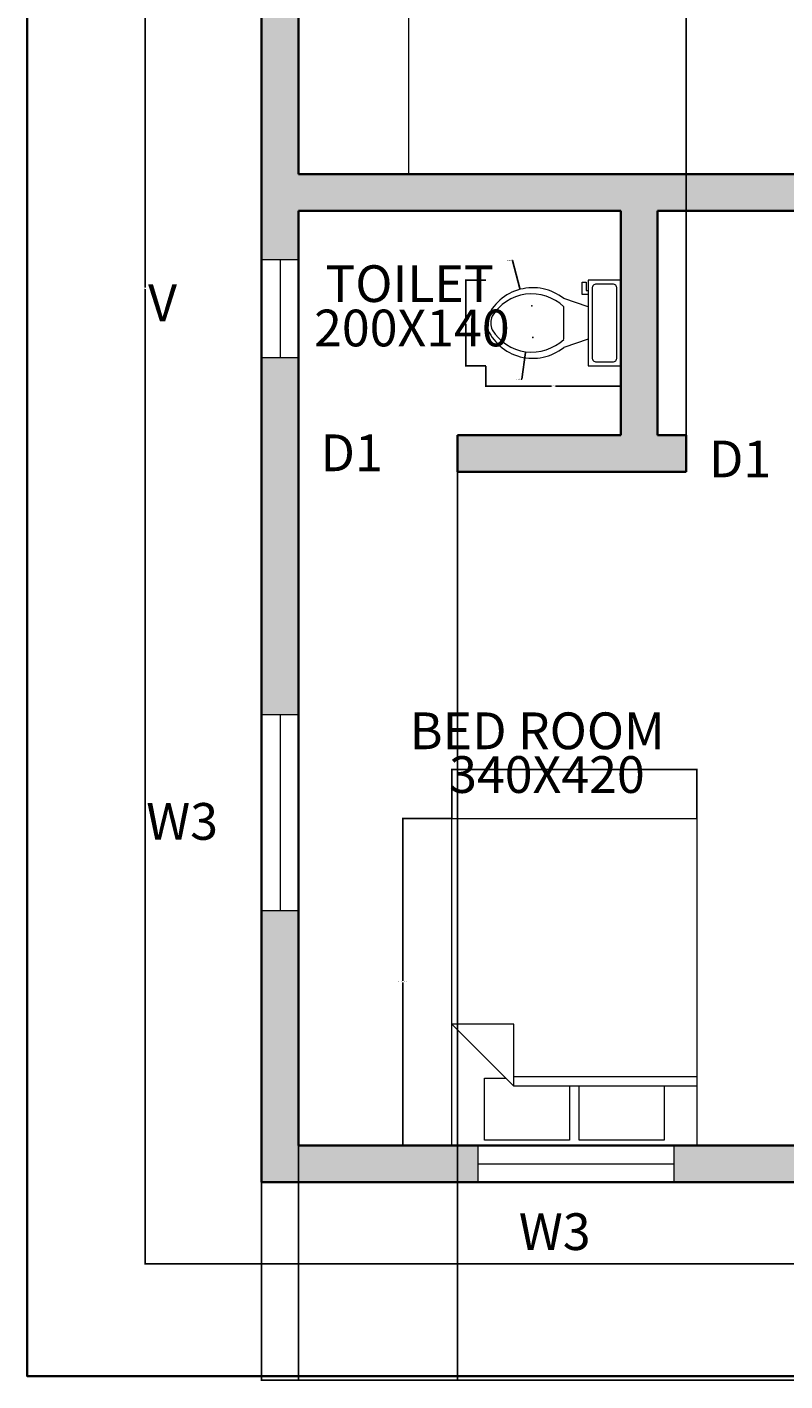
# Model space of a CAD drawing. Units: inches. Extents: x 1332 to 3175, y 1481 to 2088.
# Tile 1 of 5: x 1332 to 1518, y 1484 to 1816. Entities that reach past the tile are written whole.
import ezdxf

# ---------------------------------------------------------------- set-up
doc = ezdxf.new("R2010")
doc.units = ezdxf.units.IN
for name, color, linetype, lineweight in [('A-ANNO-DIMS', 2, 'Continuous', 18), ('A-ANNO-TEXT', 7, 'Continuous', 18), ('A-ANNO-TTLB', 7, 'Continuous', 35), ('A-AREA-IDEN', 7, 'Continuous', 18), ('A-FLOR-CASE', 8, 'Continuous', 18), ('A-FLOR-FIXT', 8, 'Continuous', 18), ('A-FURN', 8, 'Continuous', 18), ('A-WALL', 7, 'Continuous', 35)]:
    doc.layers.add(name, color=color, linetype=linetype, lineweight=lineweight)
doc.layers.add('A-GLAZ', color=30, linetype='Continuous', lineweight=18, true_color=0xf8991e)
doc.layers.add('A-WALL-PATT', color=18, linetype='Continuous', lineweight=13, true_color=0x000000)
doc.styles.get("Standard").update_dxf_attribs({"font": 'arial.ttf'})
doc.dimstyles.get("Standard").update_dxf_attribs({"dimtxt": 0.18, "dimasz": 0.18, "dimexe": 0.18, "dimexo": 0.0625, "dimgap": 0.09, "dimtad": 0, "dimtih": 1, "dimtoh": 1, "dimdec": 4, "dimzin": 0, "dimdsep": 46, "dimtxsty": 'Standard', "dimcen": 0.09, "dimadec": 0, "dimazin": 0, "dimtfac": 1, "dimtdec": 4, "dimtofl": 0, "dimtmove": 0, "dimatfit": 3, "dimfxl": 1, "dimtolj": 1, "dimtzin": 0, "dimarcsym": 0})

# ---------------------------------------------------------------- blocks, each defined once
blk = doc.blocks.new('Bed - Queen')
for p, q in [((0, -80.00003), (0, 0)), ((0, 0), (59.99999, 0)), ((59.99999, 0), (59.99999, -80.00003)), ((7.99999, -1.2), (28.79998, -1.2)), ((7.99999, -14.4), (7.99999, -1.2)), ((28.79998, -1.2), (28.79998, -14.4)), ((31.19999, -1.2), (51.99999, -1.2)), ((31.19999, -14.4), (31.19999, -1.2)), ((51.99999, -1.2), (51.99999, -16.4)), ((0, -14.4), (44.8, -14.4)), ((59.99999, -29.6), (44.8, -14.4)), ((44.8, -14.4), (44.8, -29.6)), ((51.99999, -16.4), (46.79936, -16.4)), ((44.8, -16.8), (0, -16.8)), ((44.8, -29.6), (59.99999, -29.6)), ((59.99999, -80.00003), (0, -80.00003))]:
    blk.add_line(p, q)
blk = doc.blocks.new('Toilet - top')
for p, q in [((9.5, -6), (9.5, -2)), ((-10, -8.5), (-8, -8.5)), ((-10, -9.5), (-10, -8.5)), ((-7, -9.5), (-10, -9.5)), ((-8, -8.5), (-8, -8)), ((-7, -8), (-7, -9.5)), ((-4, -8), (-6, -14)), ((4, -8), (6, -14)), ((4, -14), (-4, -14))]:
    blk.add_line(p, q)
blk.add_lwpolyline([(10.5, -8), (10.5, 0), (-10.5, 0), (-10.5, -8)], close=True)
for points in [[(-9.5, -2), (-9.5, -6)], [(8.5, -1), (-8.5, -1)], [(-8.5, -7), (8.5, -7)]]:
    blk.add_lwpolyline(points)
for centre, radius, start, end in [((-8.62, -1.88), 0.884, 81.8699, 188.1301), ((8.62, -1.88), 0.884, 351.8699, 98.1301), ((-8.62, -6.12), 0.884, 171.8699, 278.1301), ((8.62, -6.12), 0.884, 261.8699, 8.1301), ((3.52, -21.58), 12.17, 141.4691, 247.9714), ((4.2, -21.82), 11.33, 136.3677, 238.9468), ((-3.52, -21.58), 12.17, 292.0284, 38.5307), ((-4.2, -21.82), 11.33, 301.053, 43.6321), ((0, -27.88), 4, 245.7318, 294.2682), ((0, -29), 4, 254.8605, 285.1395)]:
    blk.add_arc(centre, radius, start, end)
blk = doc.blocks.new('WIN-W3-48')
for p, q in [((0, 9), (0, 0)), ((48, 9), (48, 0)), ((0, 4.5), (48, 4.5))]:
    blk.add_line(p, q)
blk = doc.blocks.new('VENT-24')
for p, q in [((0, 9), (0, 0)), ((24, 9), (24, 0)), ((0, 4.5), (24, 4.5))]:
    blk.add_line(p, q)
blk = doc.blocks.new('*D19')
at = {"layer": 'A-ANNO-DIMS', "color": 0, "lineweight": -2, "transparency": 16777216}
for p, q in [((1436.18, 1622.23), (1424.06, 1622.23)), ((1424.24, 1622.05), (1424.24, 1582.42)), ((1424.24, 1542.41), (1424.24, 1582.04)), ((1436.18, 1542.23), (1424.06, 1542.23))]:
    blk.add_line(p, q, dxfattribs=at)
at = {"layer": 'A-ANNO-DIMS', "color": 0, "transparency": 16777216}
for points in [[(1424.21, 1622.05), (1424.27, 1622.05), (1424.24, 1622.23)], [(1424.21, 1542.41), (1424.27, 1542.41), (1424.24, 1542.23)]]:
    blk.add_solid(points, dxfattribs=at)
at = {"layer": 'Defpoints', "color": 0, "transparency": 16777216}
for p in [(1436.24, 1622.23), (1424.24, 1542.23), (1436.24, 1542.23)]:
    blk.add_point(p, dxfattribs=at)
at = {"layer": 'A-ANNO-DIMS', "color": 0, "transparency": 16777216, "insert": (1424.24, 1582.23), "char_height": 0.18, "attachment_point": 5}
blk.add_mtext('\\A1;QUEEN BED 80 TYP.', dxfattribs=at)
blk = doc.blocks.new('*D20')
at = {"layer": 'A-ANNO-DIMS', "color": 0, "lineweight": -2, "transparency": 16777216}
for p, q in [((1436.24, 1622.29), (1436.24, 1634.41)), ((1436.42, 1634.23), (1465.72, 1634.23)), ((1496.06, 1634.23), (1466.77, 1634.23)), ((1496.24, 1622.29), (1496.24, 1634.41))]:
    blk.add_line(p, q, dxfattribs=at)
at = {"layer": 'A-ANNO-DIMS', "color": 0, "transparency": 16777216}
for points in [[(1436.42, 1634.26), (1436.42, 1634.2), (1436.24, 1634.23)], [(1496.06, 1634.26), (1496.06, 1634.2), (1496.24, 1634.23)]]:
    blk.add_solid(points, dxfattribs=at)
at = {"layer": 'Defpoints', "color": 0, "transparency": 16777216}
for p in [(1436.24, 1634.23), (1436.24, 1622.23), (1496.24, 1622.23)]:
    blk.add_point(p, dxfattribs=at)
at = {"layer": 'A-ANNO-DIMS', "color": 0, "transparency": 16777216, "insert": (1466.24, 1634.23), "char_height": 0.18, "attachment_point": 5}
blk.add_mtext('\\A1;60 TYP.', dxfattribs=at)
blk = doc.blocks.new('*D35')
at = {"layer": 'A-ANNO-DIMS', "color": 0, "lineweight": -2, "transparency": 16777216}
for p, q in [((1444.59, 1733.06), (1444.59, 1727.98)), ((1477.63, 1733.06), (1477.63, 1727.98)), ((1444.77, 1728.16), (1460.64, 1728.16)), ((1477.45, 1728.16), (1461.58, 1728.16))]:
    blk.add_line(p, q, dxfattribs=at)
at = {"layer": 'A-ANNO-DIMS', "color": 0, "transparency": 16777216}
for points in [[(1444.77, 1728.19), (1444.77, 1728.13), (1444.59, 1728.16)], [(1477.45, 1728.19), (1477.45, 1728.13), (1477.63, 1728.16)]]:
    blk.add_solid(points, dxfattribs=at)
at = {"layer": 'Defpoints', "color": 0, "transparency": 16777216}
for p in [(1444.59, 1733.12), (1477.63, 1733.12), (1477.63, 1728.16)]:
    blk.add_point(p, dxfattribs=at)
at = {"layer": 'A-ANNO-DIMS', "color": 0, "transparency": 16777216, "insert": (1461.11, 1728.16), "char_height": 0.18, "attachment_point": 5}
blk.add_mtext('\\A1;WC 33', dxfattribs=at)
blk = doc.blocks.new('*D36')
at = {"layer": 'A-ANNO-DIMS', "color": 0, "lineweight": -2, "transparency": 16777216}
for p, q in [((1444.52, 1754.12), (1439.45, 1754.12)), ((1439.63, 1753.94), (1439.63, 1743.8)), ((1439.63, 1733.3), (1439.63, 1743.44)), ((1444.52, 1733.12), (1439.45, 1733.12))]:
    blk.add_line(p, q, dxfattribs=at)
at = {"layer": 'A-ANNO-DIMS', "color": 0, "transparency": 16777216}
for points in [[(1439.6, 1753.94), (1439.66, 1753.94), (1439.63, 1754.12)], [(1439.6, 1733.3), (1439.66, 1733.3), (1439.63, 1733.12)]]:
    blk.add_solid(points, dxfattribs=at)
at = {"layer": 'Defpoints', "color": 0, "transparency": 16777216}
for p in [(1444.59, 1754.12), (1439.63, 1733.12), (1444.59, 1733.12)]:
    blk.add_point(p, dxfattribs=at)
at = {"layer": 'A-ANNO-DIMS', "color": 0, "transparency": 16777216, "insert": (1439.63, 1743.62), "char_height": 0.18, "attachment_point": 5}
blk.add_mtext('\\A1;21', dxfattribs=at)
blk = doc.blocks.new('*D37')
at = {"layer": 'A-ANNO-DIMS', "color": 0, "lineweight": -2, "transparency": 16777216}
for p, q in [((1851.13, 1589.06), (1851.13, 1484.44)), ((1389.63, 1533.06), (1389.63, 1484.44)), ((1389.81, 1484.62), (1619.98, 1484.62)), ((1850.95, 1484.62), (1620.78, 1484.62))]:
    blk.add_line(p, q, dxfattribs=at)
at = {"layer": 'A-ANNO-DIMS', "color": 0, "transparency": 16777216}
for points in [[(1389.81, 1484.65), (1389.81, 1484.59), (1389.63, 1484.62)], [(1850.95, 1484.65), (1850.95, 1484.59), (1851.13, 1484.62)]]:
    blk.add_solid(points, dxfattribs=at)
at = {"layer": 'Defpoints', "color": 0, "transparency": 16777216}
for p in [(1851.13, 1589.12), (1389.63, 1533.12), (1851.13, 1484.62)]:
    blk.add_point(p, dxfattribs=at)
at = {"layer": 'A-ANNO-DIMS', "color": 0, "transparency": 16777216, "insert": (1620.38, 1484.62), "char_height": 0.18, "attachment_point": 5}
blk.add_mtext('\\A1;461.5', dxfattribs=at)
blk = doc.blocks.new('*D38')
at = {"layer": 'A-ANNO-DIMS', "color": 0, "lineweight": -2, "transparency": 16777216}
for p, q in [((1444.57, 1991.12), (1360.95, 1991.12)), ((1361.13, 1990.94), (1361.13, 1752.3)), ((1361.13, 1513.3), (1361.13, 1751.94)), ((1532.57, 1513.12), (1360.95, 1513.12))]:
    blk.add_line(p, q, dxfattribs=at)
at = {"layer": 'A-ANNO-DIMS', "color": 0, "transparency": 16777216}
for points in [[(1361.1, 1990.94), (1361.16, 1990.94), (1361.13, 1991.12)], [(1361.1, 1513.3), (1361.16, 1513.3), (1361.13, 1513.12)]]:
    blk.add_solid(points, dxfattribs=at)
at = {"layer": 'Defpoints', "color": 0, "transparency": 16777216}
for p in [(1361.13, 1991.12), (1444.63, 1991.12), (1532.63, 1513.12)]:
    blk.add_point(p, dxfattribs=at)
at = {"layer": 'A-ANNO-DIMS', "color": 0, "transparency": 16777216, "insert": (1361.13, 1752.12), "char_height": 0.18, "attachment_point": 5}
blk.add_mtext('\\A1;478', dxfattribs=at)
blk = doc.blocks.new('*D86')
at = {"layer": 'A-ANNO-DIMS', "color": 0, "lineweight": -2, "transparency": 16777216}
for p, q in [((1398.63, 1735.06), (1398.63, 1484.44)), ((1437.63, 1716.06), (1437.63, 1484.44)), ((1398.81, 1484.62), (1417.91, 1484.62)), ((1437.45, 1484.62), (1418.35, 1484.62))]:
    blk.add_line(p, q, dxfattribs=at)
at = {"layer": 'A-ANNO-DIMS', "color": 0, "transparency": 16777216}
for points in [[(1398.81, 1484.65), (1398.81, 1484.59), (1398.63, 1484.62)], [(1437.45, 1484.65), (1437.45, 1484.59), (1437.63, 1484.62)]]:
    blk.add_solid(points, dxfattribs=at)
at = {"layer": 'Defpoints', "color": 0, "transparency": 16777216}
for p in [(1398.63, 1735.12), (1437.63, 1716.12), (1437.63, 1484.62)]:
    blk.add_point(p, dxfattribs=at)
at = {"layer": 'A-ANNO-DIMS', "color": 0, "transparency": 16777216, "insert": (1418.13, 1484.62), "char_height": 0.18, "attachment_point": 5}
blk.add_mtext('\\A1;39', dxfattribs=at)
blk = doc.blocks.new('*D87')
at = {"layer": 'A-ANNO-DIMS', "color": 0, "lineweight": -2, "transparency": 16777216}
for p, q in [((1493.63, 1716.18), (1493.63, 2019.8)), ((1493.81, 2019.62), (1512.91, 2019.62)), ((1532.45, 2019.62), (1513.35, 2019.62)), ((1532.63, 1716.18), (1532.63, 2019.8))]:
    blk.add_line(p, q, dxfattribs=at)
at = {"layer": 'A-ANNO-DIMS', "color": 0, "transparency": 16777216}
for points in [[(1493.81, 2019.65), (1493.81, 2019.59), (1493.63, 2019.62)], [(1532.45, 2019.65), (1532.45, 2019.59), (1532.63, 2019.62)]]:
    blk.add_solid(points, dxfattribs=at)
at = {"layer": 'Defpoints', "color": 0, "transparency": 16777216}
for p in [(1532.63, 2019.62), (1493.63, 1716.12), (1532.63, 1716.12)]:
    blk.add_point(p, dxfattribs=at)
at = {"layer": 'A-ANNO-DIMS', "color": 0, "transparency": 16777216, "insert": (1513.13, 2019.62), "char_height": 0.18, "attachment_point": 5}
blk.add_mtext('\\A1;39', dxfattribs=at)
blk = doc.blocks.new('*D92')
at = {"layer": 'A-ANNO-DIMS', "color": 0, "lineweight": -2, "transparency": 16777216}
for p, q in [((1450.92, 1758.93), (1451.1, 1758.93)), ((1451.1, 1758.93), (1452.91, 1752.04)), ((1455.96, 1740.1), (1456.14, 1740.1)), ((1456.05, 1740.01), (1456.05, 1740.19))]:
    blk.add_line(p, q, dxfattribs=at)
at = {"layer": 'A-ANNO-DIMS', "color": 0, "transparency": 16777216}
blk.add_solid([(1452.94, 1752.05), (1452.88, 1752.03), (1452.96, 1751.87)], dxfattribs=at)
at = {"layer": 'Defpoints', "color": 0, "transparency": 16777216}
for p in [(1452.96, 1751.87), (1456.05, 1740.1)]:
    blk.add_point(p, dxfattribs=at)
at = {"layer": 'A-ANNO-DIMS', "color": 0, "transparency": 16777216, "insert": (1450.25, 1758.93), "char_height": 0.18, "attachment_point": 5}
blk.add_mtext('\\A1;2X R12.17', dxfattribs=at)
blk = doc.blocks.new('*D93')
at = {"layer": 'A-ANNO-DIMS', "color": 0, "lineweight": -2, "transparency": 16777216}
for p, q in [((1455.72, 1747.82), (1455.9, 1747.82)), ((1455.81, 1747.73), (1455.81, 1747.91)), ((1453.4, 1729.85), (1454.28, 1736.41)), ((1453.22, 1729.85), (1453.4, 1729.85))]:
    blk.add_line(p, q, dxfattribs=at)
at = {"layer": 'A-ANNO-DIMS', "color": 0, "transparency": 16777216}
blk.add_solid([(1454.25, 1736.42), (1454.31, 1736.41), (1454.3, 1736.59)], dxfattribs=at)
at = {"layer": 'Defpoints', "color": 0, "transparency": 16777216}
for p in [(1455.81, 1747.82), (1454.3, 1736.59)]:
    blk.add_point(p, dxfattribs=at)
at = {"layer": 'A-ANNO-DIMS', "color": 0, "transparency": 16777216, "insert": (1452.54, 1729.85), "char_height": 0.18, "attachment_point": 5}
blk.add_mtext('\\A1;2X R11.33', dxfattribs=at)

msp = doc.modelspace()

# ---------------------------------------------------------------- hatches: boundary and pattern name
at = {"layer": 'A-WALL-PATT'}
h = msp.add_hatch(color=256, dxfattribs=at)
h.dxf.hatch_style = 1
h.paths.add_polyline_path([(1398.6316, 1914.1183), (1442.6316, 1914.1183), (1442.6316, 1923.1183), (1389.6316, 1923.1183), (1389.6316, 1868.1183), (1398.6316, 1868.1183)])
h.paths.add_polyline_path([(1398.6316, 1828.1183), (1389.6316, 1828.1183), (1389.6316, 1759.1183), (1398.6316, 1759.1183), (1398.6316, 1771.1183), (1477.6316, 1771.1183), (1477.6316, 1716.1183), (1437.6316, 1716.1183), (1437.6316, 1707.1183), (1493.6316, 1707.1183), (1493.6316, 1716.1183), (1486.6316, 1716.1183), (1486.6316, 1771.1183), (1532.6316, 1771.1183), (1532.6316, 1780.1183), (1398.6316, 1780.1183)])
h.paths.add_polyline_path([(1398.6316, 1735.1183), (1389.6316, 1735.1183), (1389.6316, 1647.6183), (1398.6316, 1647.6183)])
h.paths.add_polyline_path([(1398.6316, 1599.6183), (1389.6316, 1599.6183), (1389.6316, 1533.1183), (1442.6316, 1533.1183), (1442.6316, 1542.1183), (1398.6316, 1542.1183)])
h.paths.add_polyline_path([(1541.6316, 1589.1183), (1576.5616, 1589.1183), (1576.5616, 1598.1183), (1541.6316, 1598.1183), (1541.6316, 1707.1183), (1576.5616, 1707.1183), (1576.5616, 1716.1183), (1532.6316, 1716.1183), (1532.6316, 1542.1183), (1490.6316, 1542.1183), (1490.6316, 1533.1183), (1541.6316, 1533.1183)])
h.paths.add_polyline_path([(1717.1316, 1707.1183), (1752.1316, 1707.1183), (1752.1316, 1716.1183), (1672.5616, 1716.1183), (1672.5616, 1707.1183), (1708.1316, 1707.1183), (1708.1316, 1598.1183), (1672.5616, 1598.1183), (1672.5616, 1589.1183), (1717.1316, 1589.1183)])
h.paths.add_polyline_path([(1851.1316, 1761.1183), (1842.1316, 1761.1183), (1842.1316, 1716.1183), (1800.1316, 1716.1183), (1800.1316, 1707.1183), (1851.1316, 1707.1183)])
h.paths.add_polyline_path([(1851.1316, 1855.1183), (1784.1316, 1855.1183), (1784.1316, 1923.1183), (1750.1316, 1923.1183), (1750.1316, 1914.1183), (1775.1316, 1914.1183), (1775.1316, 1855.1183), (1750.1316, 1855.1183), (1750.1316, 1846.1183), (1842.1316, 1846.1183), (1842.1316, 1801.1183), (1851.1316, 1801.1183)])
h.paths.add_polyline_path([(1717.1316, 1914.1183), (1726.1316, 1914.1183), (1726.1316, 1923.1183), (1673.1316, 1923.1183), (1673.1316, 1914.1183), (1708.1316, 1914.1183), (1708.1316, 1755.1183), (1717.1316, 1755.1183)])
h.paths.add_polyline_path([(1661.1316, 1855.1183), (1636.1316, 1855.1183), (1636.1316, 1914.1183), (1649.1316, 1914.1183), (1649.1316, 1923.1183), (1611.3665, 1923.1183), (1611.3665, 1914.1183), (1627.1316, 1914.1183), (1627.1316, 1846.1183), (1661.1316, 1846.1183)])
h.paths.add_polyline_path([(1541.6316, 1914.1183), (1563.3665, 1914.1183), (1563.3665, 1923.1183), (1541.6316, 1923.1183), (1541.6316, 1991.1183), (1528.6316, 1991.1183), (1528.6316, 1982.1183), (1532.6316, 1982.1183), (1532.6316, 1914.1183), (1532.6316, 1816.1183), (1541.6316, 1816.1183)])
h.paths.add_polyline_path([(1453.6316, 1982.1183), (1457.6316, 1982.1183), (1457.6316, 1991.1183), (1444.6316, 1991.1183), (1444.6316, 1956.1183), (1453.6316, 1956.1183)])

# ---------------------------------------------------------------- linework, layer by layer
at = {"layer": 'A-ANNO-TTLB'}
msp.add_lwpolyline([(1332.1674, 2088.4777), (3159.6908, 2088.4777), (3159.6908, 1485.6439), (1332.1674, 1485.6439)], close=True, dxfattribs=at)
at = {"layer": 'A-FLOR-CASE'}
msp.add_line((1425.7005, 1780.1183), (1425.7005, 1891.601), dxfattribs=at)
at = {"layer": 'A-WALL'}
for p, q in [((1389.6316, 1923.1183), (1389.6316, 1533.1183)), ((1398.6316, 1914.1183), (1398.6316, 1780.1183)), ((1398.6316, 1780.1183), (1532.6316, 1780.1183)), ((1398.6316, 1771.1183), (1477.6316, 1771.1183)), ((1398.6316, 1771.1183), (1398.6316, 1542.1183)), ((1477.6316, 1771.1183), (1477.6316, 1716.1183)), ((1486.6316, 1771.1183), (1486.6316, 1716.1183)), ((1486.6316, 1771.1183), (1532.6316, 1771.1183)), ((1437.6316, 1716.1183), (1477.6316, 1716.1183)), ((1437.6316, 1716.1183), (1477.6316, 1716.1183)), ((1437.6316, 1716.1183), (1437.6316, 1707.1183)), ((1486.6316, 1716.1183), (1493.6316, 1716.1183)), ((1486.6316, 1716.1183), (1493.6316, 1716.1183)), ((1493.6316, 1716.1183), (1493.6316, 1707.1183)), ((1437.6316, 1707.1183), (1493.6316, 1707.1183)), ((1398.6316, 1542.1183), (1532.6316, 1542.1183)), ((1389.6316, 1533.1183), (1541.6316, 1533.1183))]:
    msp.add_line(p, q, dxfattribs=at)

# ---------------------------------------------------------------- block references
at = {"layer": 'A-FLOR-FIXT', "rotation": 270}
msp.add_blockref('Toilet - top', (1477.6316, 1743.6183), dxfattribs=at)
at = {"layer": 'A-FURN', "rotation": 180}
msp.add_blockref('Bed - Queen', (1496.2447, 1542.2313), dxfattribs=at)
at = {"layer": 'A-GLAZ'}
for name, p, rotation in [('VENT-24', (1389.6316, 1759.1183), 270.0000000000015), ('WIN-W3-48', (1389.6316, 1647.6183), 270.0000000000006)]:
    msp.add_blockref(name, p, dxfattribs=dict(at, rotation=rotation))
msp.add_blockref('WIN-W3-48', (1442.6316, 1533.1183), dxfattribs=at)

# ---------------------------------------------------------------- texts
at = {"layer": 'A-ANNO-TEXT'}
for s, p in [('      V', (1345.3144, 1744.0608)), ('      D1', (1387.5429, 1707.3201)), ('      D1', (1482.7043, 1705.8048)), ('    W3', (1350.3492, 1617.0164)), ('    W3', (1441.6235, 1516.511))]:
    msp.add_text(s, height=9, dxfattribs=at).set_placement(p)
at = {"layer": 'A-AREA-IDEN'}
for s, p in [(' TOILET', (1402.4712, 1748.759)), ('200X140', (1402.4712, 1737.8945)), ('BED ROOM', (1425.8978, 1639.2106)), ('340X420', (1435.5603, 1628.4969))]:
    msp.add_text(s, height=9, dxfattribs=at).set_placement(p)

# ---------------------------------------------------------------- dimensions: what is measured, and where the dimension line sits
at = {"layer": 'A-ANNO-DIMS'}
for base, p1, p2, override, picture, middle in [((1532.6316, 2019.6183), (1493.6316, 1716.1183), (1532.6316, 1716.1183), {"dimdec": 0, "dimlfac": 1, "dimrnd": 0, "dimzin": 0, "dimdsep": 46, "dimlunit": 2}, '*D87', (1513.1316, 2019.6183)), ((1437.6316, 1484.6183), (1398.6316, 1735.1183), (1437.6316, 1716.1183), {"dimdec": 0, "dimlfac": 1, "dimrnd": 0, "dimzin": 0, "dimdsep": 46, "dimlunit": 2}, '*D86', (1418.1316, 1484.6183)), ((1851.1316, 1484.6183), (1389.6316, 1533.1183), (1851.1316, 1589.1183), {"dimdec": 1, "dimlfac": 1, "dimrnd": 0, "dimzin": 0, "dimdsep": 46, "dimlunit": 2}, '*D37', (1620.3816, 1484.6183))]:
    dim = msp.add_linear_dim(base=base, p1=p1, p2=p2, dimstyle='Standard', override=override, dxfattribs=at)
    dim.commit()
    dim.dimension.update_dxf_attribs({"geometry": picture, "text_midpoint": middle})
for base, p1, p2, angle, picture, middle in [((1361.1316, 1991.1183), (1532.6316, 1513.1183), (1444.6316, 1991.1183), 90, '*D38', (1361.1316, 1752.1183)), ((1439.6284, 1733.1183), (1444.5853, 1754.1183), (1444.5853, 1733.1183), 270, '*D36', (1439.6284, 1743.6183))]:
    dim = msp.add_linear_dim(base=base, p1=p1, p2=p2, angle=angle, dimstyle='Standard', override={"dimdec": 0, "dimlfac": 1, "dimrnd": 0, "dimzin": 0, "dimdsep": 46, "dimlunit": 2}, dxfattribs=at)
    dim.commit()
    dim.dimension.update_dxf_attribs({"geometry": picture, "text_midpoint": middle})
for center, mpoint, picture, middle in [((1456.0511, 1740.0987), (1452.9589, 1751.8683), '*D92', (1450.2489, 1758.9301)), ((1455.8142, 1747.8181), (1454.305, 1736.5899), '*D93', (1452.5447, 1729.853))]:
    dim = msp.add_radius_dim(center=center, mpoint=mpoint, text='2X <>', dimstyle='Standard', override={"dimdec": 2, "dimlfac": 1, "dimrnd": 0, "dimzin": 0, "dimdsep": 46, "dimlunit": 2}, dxfattribs=at)
    dim.commit()
    dim.dimension.update_dxf_attribs({"geometry": picture, "text_midpoint": middle, "dimtype": 164})
dim = msp.add_linear_dim(base=(1477.6316, 1728.1613), p1=(1444.5853, 1733.1183), p2=(1477.6316, 1733.1183), text='WC <>', dimstyle='Standard', override={"dimdec": 0, "dimlfac": 1, "dimrnd": 0, "dimzin": 0, "dimdsep": 46, "dimlunit": 2}, dxfattribs=at)
dim.commit()
dim.dimension.update_dxf_attribs({"geometry": '*D35', "text_midpoint": (1461.1085, 1728.1613)})
for base, p1, p2, angle, text, picture, middle in [((1436.2447, 1634.2313), (1496.2447, 1622.2313), (1436.2447, 1622.2313), 180, '<> TYP.', '*D20', (1466.2447, 1634.2313)), ((1424.2447, 1542.2313), (1436.2447, 1622.2313), (1436.2447, 1542.2313), 270, 'QUEEN BED <> TYP.', '*D19', (1424.2447, 1582.2313))]:
    dim = msp.add_linear_dim(base=base, p1=p1, p2=p2, angle=angle, text=text, dimstyle='Standard', override={"dimdec": 0, "dimlfac": 1, "dimrnd": 0, "dimzin": 0, "dimdsep": 46, "dimlunit": 2}, dxfattribs=at)
    dim.commit()
    dim.dimension.update_dxf_attribs({"geometry": picture, "text_midpoint": middle})

doc.saveas('drawing.dxf')
